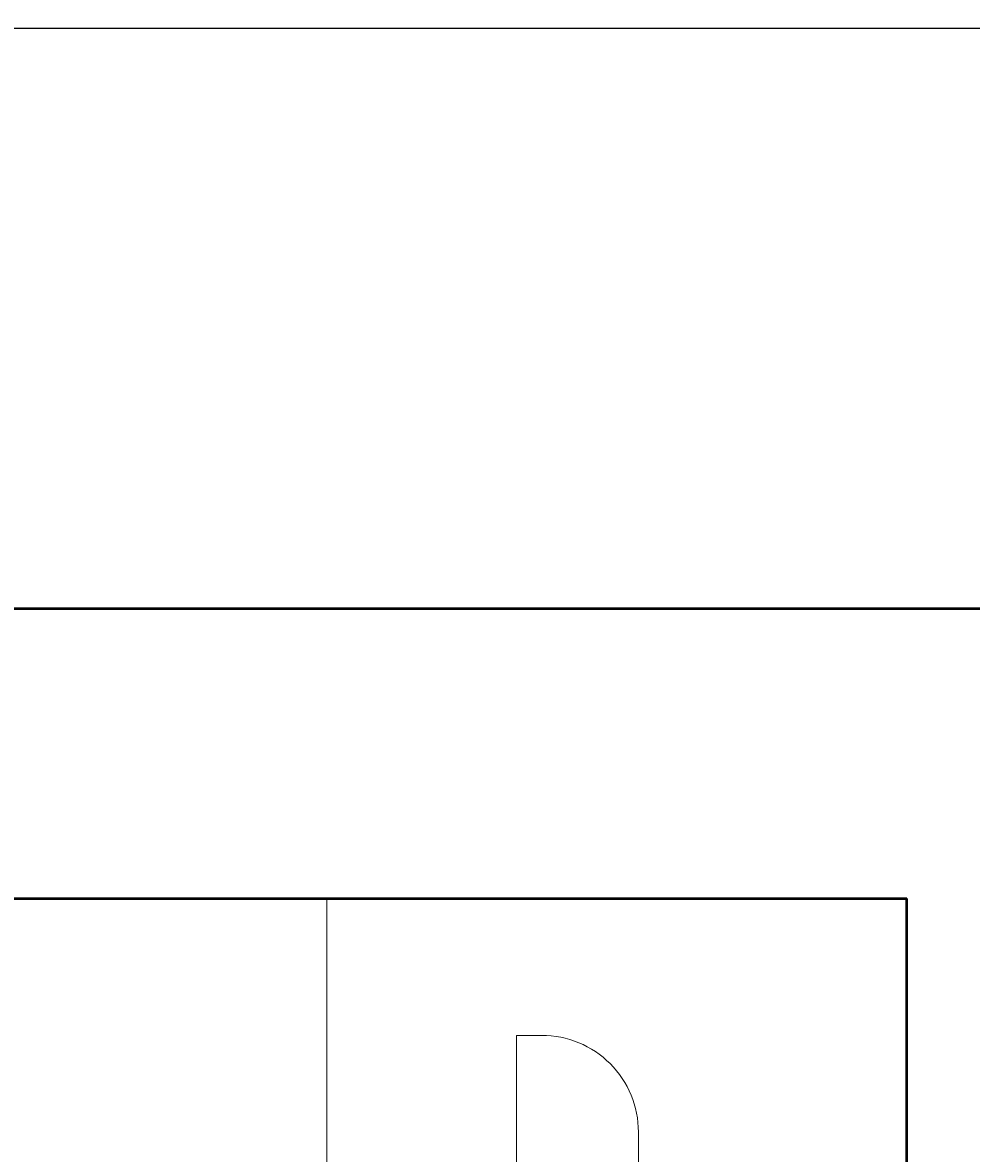
# Model space of a CAD drawing. Units: inches. Extents: x 2621 to 2849, y 2066 to 2463.
# Tile 19 of 28: x 2736 to 2766, y 2427 to 2463. Entities that reach past the tile are written whole.
import ezdxf

# ---------------------------------------------------------------- set-up
doc = ezdxf.new("R2010")
doc.units = ezdxf.units.IN
for name, color, linetype, lineweight in [('A-ANNO-DIMS', 2, 'Continuous', 18), ('A-EQPM', 8, 'Continuous', 18), ('A-FURN', 8, 'Continuous', 18), ('A-WALL', 7, 'Continuous', 50)]:
    doc.layers.add(name, color=color, linetype=linetype, lineweight=lineweight)
doc.styles.get("Standard").update_dxf_attribs({"font": 'arial.ttf'})
doc.dimstyles.get("Standard").update_dxf_attribs({"dimtxt": 0.18, "dimasz": 0.18, "dimexe": 0.18, "dimexo": 0.0625, "dimgap": 0.09, "dimtad": 0, "dimtih": 1, "dimtoh": 1, "dimdec": 4, "dimzin": 0, "dimdsep": 46, "dimtxsty": 'Standard', "dimcen": 0.09, "dimadec": 0, "dimazin": 0, "dimtfac": 1, "dimtdec": 4, "dimtofl": 0, "dimtmove": 0, "dimatfit": 3, "dimfxl": 1, "dimtolj": 1, "dimtzin": 0, "dimarcsym": 0})

# ---------------------------------------------------------------- blocks, each defined once
blk = doc.blocks.new('*D35')
at = {"layer": 'A-ANNO-DIMS', "color": 0, "lineweight": -2, "transparency": 16777216}
for p, q in [((2638.87, 2444.437), (2638.87, 2462.558)), ((2830.87, 2444.437), (2830.87, 2462.558)), ((2639.05, 2462.378), (2734.591, 2462.378)), ((2830.69, 2462.378), (2735.15, 2462.378))]:
    blk.add_line(p, q, dxfattribs=at)
at = {"layer": 'A-ANNO-DIMS', "color": 0, "transparency": 16777216}
for points in [[(2639.05, 2462.408), (2639.05, 2462.348), (2638.87, 2462.378)], [(2830.69, 2462.408), (2830.69, 2462.348), (2830.87, 2462.378)]]:
    blk.add_solid(points, dxfattribs=at)
at = {"layer": 'Defpoints', "color": 0, "transparency": 16777216}
for p in [(2830.87, 2462.378), (2638.87, 2444.375), (2830.87, 2444.375)]:
    blk.add_point(p, dxfattribs=at)
at = {"layer": 'A-ANNO-DIMS', "color": 0, "transparency": 16777216, "insert": (2734.87, 2462.378), "char_height": 0.18, "attachment_point": 5}
blk.add_mtext('\\A1;192', dxfattribs=at)
blk = doc.blocks.new('*D68')
at = {"layer": 'A-ANNO-DIMS', "color": 0, "lineweight": -2, "transparency": 16777216}
for p, q in [((2745.808, 2435.375), (2620.687, 2435.375)), ((2620.867, 2435.195), (2620.867, 2405.556)), ((2620.867, 2375.555), (2620.867, 2405.193)), ((2745.808, 2375.375), (2620.687, 2375.375))]:
    blk.add_line(p, q, dxfattribs=at)
at = {"layer": 'A-ANNO-DIMS', "color": 0, "transparency": 16777216}
for points in [[(2620.837, 2435.195), (2620.897, 2435.195), (2620.867, 2435.375)], [(2620.837, 2375.555), (2620.897, 2375.555), (2620.867, 2375.375)]]:
    blk.add_solid(points, dxfattribs=at)
at = {"layer": 'Defpoints', "color": 0, "transparency": 16777216}
for p in [(2620.867, 2435.375), (2745.87, 2435.375), (2745.87, 2375.375)]:
    blk.add_point(p, dxfattribs=at)
at = {"layer": 'A-ANNO-DIMS', "color": 0, "transparency": 16777216, "insert": (2620.867, 2405.375), "char_height": 0.18, "attachment_point": 5}
blk.add_mtext('\\A1;60', dxfattribs=at)

msp = doc.modelspace()

# ---------------------------------------------------------------- linework, layer by layer
at = {"layer": 'A-EQPM'}
msp.add_lwpolyline([(2751.7541, 2431.1293), (2752.5373, 2431.1293, -0.4142136), (2755.5373, 2428.1293), (2755.5373, 2384.6294, -0.4142136), (2752.5373, 2381.6294), (2751.7541, 2381.6294)], format="xyb", close=True, dxfattribs=at)
at = {"layer": 'A-FURN'}
msp.add_lwpolyline([(2763.8701, 2435.3746), (2745.8701, 2435.3746), (2745.8701, 2375.3746), (2763.8701, 2375.3746)], close=True, dxfattribs=at)
at = {"layer": 'A-WALL'}
for p in [(2647.8701, 2435.3746), (2763.8701, 2355.3746)]:
    msp.add_line(p, (2763.8701, 2435.3746), dxfattribs=at)
msp.add_lwpolyline([(2761.8701, 2084.3746), (2638.8701, 2084.3746), (2638.8701, 2444.3746), (2830.8701, 2444.3746), (2830.8701, 2084.3746), (2797.8701, 2084.3746)], dxfattribs=at)

# ---------------------------------------------------------------- dimensions: what is measured, and where the dimension line sits
at = {"layer": 'A-ANNO-DIMS'}
dim = msp.add_linear_dim(base=(2830.8701, 2462.3781), p1=(2638.8701, 2444.3746), p2=(2830.8701, 2444.3746), dimstyle='Standard', override={"dimdec": 0, "dimlfac": 1, "dimrnd": 0, "dimzin": 0, "dimdsep": 46, "dimlunit": 2}, dxfattribs=at)
dim.commit()
dim.dimension.update_dxf_attribs({"geometry": '*D35', "text_midpoint": (2734.8701, 2462.3781)})
dim = msp.add_linear_dim(base=(2620.8666, 2435.3746), p1=(2745.8701, 2375.3746), p2=(2745.8701, 2435.3746), angle=90, dimstyle='Standard', override={"dimdec": 0, "dimlfac": 1, "dimrnd": 0, "dimzin": 0, "dimdsep": 46, "dimlunit": 2}, dxfattribs=at)
dim.commit()
dim.dimension.update_dxf_attribs({"geometry": '*D68', "text_midpoint": (2620.8666, 2405.3746)})

doc.saveas('drawing.dxf')
